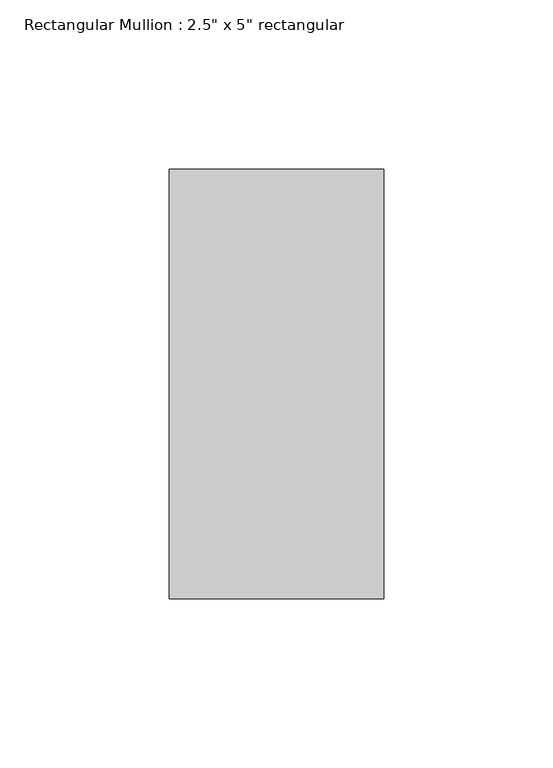
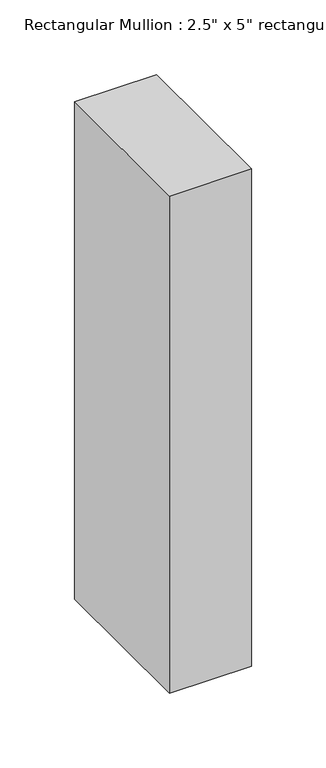
"""IFC4 building model written with IfcOpenShell, lengths in millimetres: member geometry."""

from ifc_helpers import new_model, si_unit, frame, origin, place, context, project, spatial, polyline, outline, extrude, source, transform, mapped, element, save


def member_90c805a2(model_context):
    return source(origin(), model_context, "Body", "SweptSolid", [
        extrude(outline(polyline([(31.75, 63.5), (31.75, -63.5), (-31.75, -63.5), (-31.75, 63.5), (31.75, 63.5)])), frame((0.0, 0.0, -406.4), z_axis=(0.0, 0.0, 1.0), x_axis=(1.0, 0.0, 0.0)), (0.0, 0.0, 1.0), 406.4),
    ])


if __name__ == "__main__":
    model = new_model("IFC4")
    model_context = context("Model", 3, world=origin())
    ifc_project = project(units=[si_unit("LENGTHUNIT", "METRE", prefix="MILLI")], contexts=[model_context])
    site = spatial("IfcSite", under=ifc_project)
    building = spatial("IfcBuilding", under=site)
    placement = place(None, origin())
    member_shape = member_90c805a2(model_context)
    element("IfcMember", 1, ObjectType="Rectangular Mullion : 2.5\" x 5\" rectangular", at=placement, inside=building, context=model_context, shape_type="MappedRepresentation", body=[
        mapped(member_shape, transform((0.0, 0.0, 0.0), x_axis=(1.0, 0.0, 0.0), y_axis=(0.0, 1.0, 0.0), z_axis=(0.0, 0.0, 1.0))),
    ])
    save(model, "model.ifc")

# Revit data of these elements
# Type "Rectangular Mullion : 2.5\" x 5\" rectangular"
#   built-in parameter 1007304 = 0.416667 (stored number, unit not read)
#   built-in parameter 1007301 = 0.104167 (stored number, unit not read)
#   built-in parameter 1007300 = 0.104167 (stored number, unit not read)
# Element 1 (IfcMember, "Rectangular Mullion : 2.5\" x 5\" rectangular")
#   Materials on its faces: "Aluminum"
# Materials
#   "Aluminum": class "Metal", colour RGB 247 247 247, transparency 0, Description = "Aluminum 6061", Cost = 0
